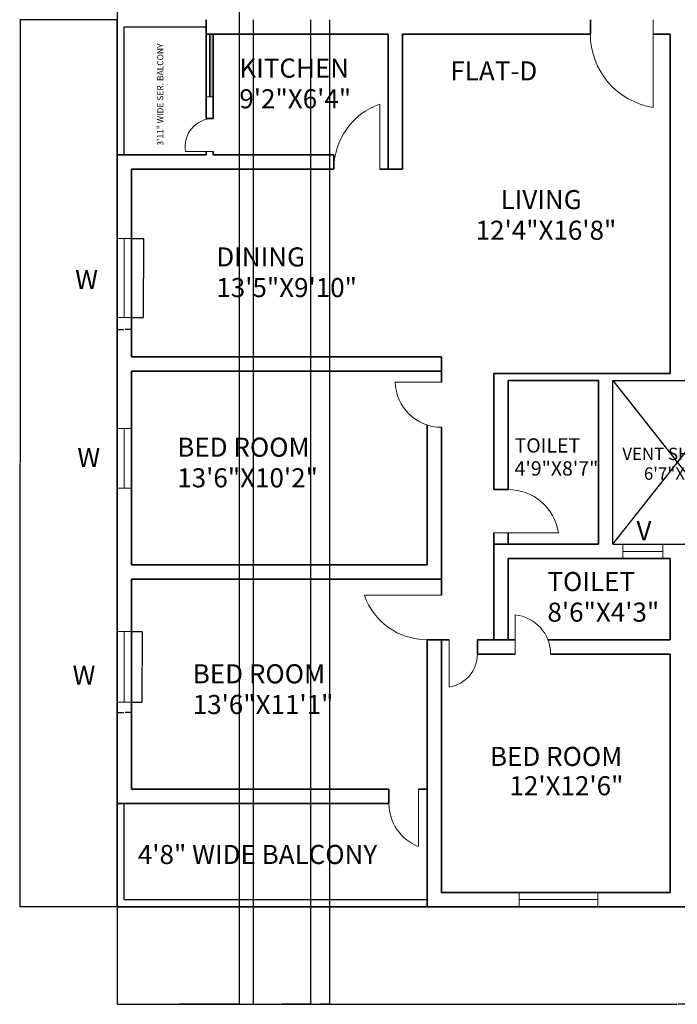
# Model space of a CAD drawing. Units: feet. Extents: x 5816 to 6644, y 25475 to 26788.
# Tile 1 of 23: x 5816 to 6230, y 25475 to 26094. Entities that reach past the tile are written whole.
import ezdxf

# ---------------------------------------------------------------- set-up
doc = ezdxf.new("R2010")
doc.units = ezdxf.units.FT
for name, color, linetype, lineweight in [('A-ANNO-DIMS', 2, 'Continuous', 13), ('A-ANNO-TEXT', 7, 'Continuous', 18), ('A-AREA-IDEN', 7, 'Continuous', 18), ('A-DOOR', 3, 'Continuous', 18), ('A-FLOR-RAIL', 8, 'Continuous', 25), ('A-FLOR-SHFT', 8, 'Continuous', 25), ('A-GLAZ', 4, 'Continuous', 18), ('A-WALL', 7, 'Continuous', 35)]:
    doc.layers.add(name, color=color, linetype=linetype, lineweight=lineweight)
doc.styles.get("Standard").update_dxf_attribs({"font": 'arial.ttf'})
doc.dimstyles.get("Standard").update_dxf_attribs({"dimtxt": 0.18, "dimasz": 0.18, "dimexe": 0.18, "dimexo": 0.0625, "dimgap": 0.09, "dimtad": 0, "dimtih": 1, "dimtoh": 1, "dimdec": 4, "dimzin": 0, "dimdsep": 46, "dimtxsty": 'Standard', "dimcen": 0.09, "dimadec": 0, "dimazin": 0, "dimtfac": 1, "dimtdec": 4, "dimtofl": 0, "dimtmove": 0, "dimatfit": 3, "dimfxl": 1, "dimtolj": 1, "dimtzin": 0, "dimarcsym": 0})

# ---------------------------------------------------------------- blocks, each defined once
blk = doc.blocks.new('DOOR-BALCONY')
blk.add_line((0, 36.11), (0, 0))
blk.add_arc((10.54, 9), 29.09, 111.24329, 180)
blk = doc.blocks.new('DOOR-BEDROOM-INNER')
blk.add_line((0, 29.82), (0, 0))
blk.add_arc((-3.45, 9), 21.11, 0, 80.59123)
blk = doc.blocks.new('DOOR-BEDROOM-BALCONY')
blk.add_line((-48.41, 0), (0, 0))
blk.add_arc((-9, -13.73), 41.74, 90, 160.78776)
blk = doc.blocks.new('DOOR-BEDROOM-SIDE')
blk.add_line((-28.98, 0), (0, 0))
blk.add_arc((0.03, -0.75), 29.02, 90, 178.52212)
blk = doc.blocks.new('DOOR-KITCHEN')
blk.add_line((0, -40.87), (0, 0))
blk.add_arc((14.45, 0), 43.35, 180, 250.52864)
blk = doc.blocks.new('DOOR-SERVICE-BALCONY')
blk.add_line((-17.56, 0), (0, 0))
blk.add_arc((0, -2.91), 17.8, 170.58679, 270)
blk = doc.blocks.new('DOOR-FLAT-ENTRY')
blk.add_line((0, 55.13), (0, 0))
blk.add_arc((7.05, 9.01), 46.66, 98.693, 180)
blk = doc.blocks.new('DOOR-BATH-ENSUITE')
blk.add_line((0, -24.59), (0, 0))
blk.add_arc((-2.33, 0.02), 24.72, 275.40734, 0)
blk = doc.blocks.new('DOOR-BATH-HALL')
blk.add_line((40.72, 0), (0, 0))
blk.add_arc((9, 4.86), 32.09, 270, 351.28818)
blk = doc.blocks.new('WIN-DINING')
for p, q in [((0, 0), (9, 0)), ((4.5, 0), (4.5, -49.84)), ((0, -49.84), (9, -49.84))]:
    blk.add_line(p, q)
blk = doc.blocks.new('WIN-BEDROOM-SIDE')
for p, q in [((0, 0), (9, 0)), ((4.5, 0), (4.5, -37.54)), ((0, -37.54), (9, -37.54))]:
    blk.add_line(p, q)
blk = doc.blocks.new('WIN-BEDROOM-BALCONY')
for p, q in [((0, 0), (9, 0)), ((4.5, 0), (4.5, -44.28)), ((0, -44.28), (9, -44.28))]:
    blk.add_line(p, q)
blk = doc.blocks.new('WIN-BEDROOM-INNER')
for p, q in [((49.5, 0), (49.5, -9)), ((0, 0), (0, -9)), ((0, -4.5), (49.5, -4.5))]:
    blk.add_line(p, q)
blk = doc.blocks.new('WIN-KITCHEN')
for p, q in [((0, 0), (4.5, 0)), ((2, 0), (2, -39.61)), ((3, 0), (3, -39.61))]:
    blk.add_line(p, q)
blk = doc.blocks.new('WIN-VENT-WIDE')
for p, q in [((0, 0), (0, -9)), ((0, -4.5), (25.2, -4.5)), ((25.2, 0), (25.2, -9))]:
    blk.add_line(p, q)
blk = doc.blocks.new('VENT-SHAFT')
for p, q in [((0, 0), (0, 103)), ((0, 103), (81, 103)), ((0, 103), (81, 0)), ((0, 0), (81, 103)), ((81, 103), (45, 103)), ((81, 0), (81, 103)), ((0, 0), (81, 0)), ((81, 0), (45, 0))]:
    blk.add_line(p, q)
blk = doc.blocks.new('RAIL-BALCONY-CORNER')
for p, q in [((0, 0), (0, -65)), ((0, 0), (195, 0)), ((4.5, -4.5), (4.5, -65)), ((4.5, -4.5), (195, -4.5))]:
    blk.add_line(p, q)
blk = doc.blocks.new('*D37')
at = {"layer": 'A-ANNO-DIMS', "color": 0, "lineweight": -2, "transparency": 16777216}
for p, q in [((5886.37, 25956.79), (5893.97, 25956.79)), ((5893.79, 25956.61), (5893.79, 25932.05)), ((5893.79, 25907.12), (5893.79, 25931.68)), ((5886.37, 25906.94), (5893.97, 25906.94))]:
    blk.add_line(p, q, dxfattribs=at)
at = {"layer": 'A-ANNO-DIMS', "color": 0, "transparency": 16777216}
for points in [[(5893.76, 25956.61), (5893.82, 25956.61), (5893.79, 25956.79)], [(5893.76, 25907.12), (5893.82, 25907.12), (5893.79, 25906.94)]]:
    blk.add_solid(points, dxfattribs=at)
at = {"layer": 'Defpoints', "color": 0, "transparency": 16777216}
for p in [(5886.31, 25956.79), (5886.31, 25906.94), (5893.79, 25906.94)]:
    blk.add_point(p, dxfattribs=at)
at = {"layer": 'A-ANNO-DIMS', "color": 0, "transparency": 16777216, "insert": (5893.79, 25931.86), "char_height": 0.18, "attachment_point": 5}
blk.add_mtext('\\A1;DINING WDW 50 TYP.', dxfattribs=at)
blk = doc.blocks.new('*D38')
at = {"layer": 'A-ANNO-DIMS', "color": 0, "lineweight": -2, "transparency": 16777216}
for p, q in [((5877.31, 25906.88), (5877.31, 25899.28)), ((5886.31, 25906.88), (5886.31, 25899.28)), ((5877.49, 25899.46), (5881.35, 25899.46)), ((5886.13, 25899.46), (5882.27, 25899.46))]:
    blk.add_line(p, q, dxfattribs=at)
at = {"layer": 'A-ANNO-DIMS', "color": 0, "transparency": 16777216}
for points in [[(5877.49, 25899.49), (5877.49, 25899.43), (5877.31, 25899.46)], [(5886.13, 25899.49), (5886.13, 25899.43), (5886.31, 25899.46)]]:
    blk.add_solid(points, dxfattribs=at)
at = {"layer": 'Defpoints', "color": 0, "transparency": 16777216}
for p in [(5877.31, 25906.94), (5886.31, 25906.94), (5877.31, 25899.46)]:
    blk.add_point(p, dxfattribs=at)
at = {"layer": 'A-ANNO-DIMS', "color": 0, "transparency": 16777216, "insert": (5881.81, 25899.46), "char_height": 0.18, "attachment_point": 5}
blk.add_mtext('\\A1;9 TYP.', dxfattribs=at)
blk = doc.blocks.new('*D41')
at = {"layer": 'A-ANNO-DIMS', "color": 0, "lineweight": -2, "transparency": 16777216}
for p, q in [((5886.37, 25709.41), (5893.13, 25709.41)), ((5892.95, 25709.23), (5892.95, 25687.45)), ((5892.95, 25665.31), (5892.95, 25687.09)), ((5886.37, 25665.13), (5893.13, 25665.13))]:
    blk.add_line(p, q, dxfattribs=at)
at = {"layer": 'A-ANNO-DIMS', "color": 0, "transparency": 16777216}
for points in [[(5892.92, 25709.23), (5892.98, 25709.23), (5892.95, 25709.41)], [(5892.92, 25665.31), (5892.98, 25665.31), (5892.95, 25665.13)]]:
    blk.add_solid(points, dxfattribs=at)
at = {"layer": 'Defpoints', "color": 0, "transparency": 16777216}
for p in [(5886.31, 25709.41), (5886.31, 25665.13), (5892.95, 25665.13)]:
    blk.add_point(p, dxfattribs=at)
at = {"layer": 'A-ANNO-DIMS', "color": 0, "transparency": 16777216, "insert": (5892.95, 25687.27), "char_height": 0.18, "attachment_point": 5}
blk.add_mtext('\\A1;BALCONY BR WDW 44 TYP.', dxfattribs=at)
blk = doc.blocks.new('*D42')
at = {"layer": 'A-ANNO-DIMS', "color": 0, "lineweight": -2, "transparency": 16777216}
for p, q in [((5877.31, 25665.07), (5877.31, 25658.31)), ((5886.31, 25665.07), (5886.31, 25658.31)), ((5877.49, 25658.49), (5881.35, 25658.49)), ((5886.13, 25658.49), (5882.27, 25658.49))]:
    blk.add_line(p, q, dxfattribs=at)
at = {"layer": 'A-ANNO-DIMS', "color": 0, "transparency": 16777216}
for points in [[(5877.49, 25658.52), (5877.49, 25658.46), (5877.31, 25658.49)], [(5886.13, 25658.52), (5886.13, 25658.46), (5886.31, 25658.49)]]:
    blk.add_solid(points, dxfattribs=at)
at = {"layer": 'Defpoints', "color": 0, "transparency": 16777216}
for p in [(5877.31, 25665.13), (5886.31, 25665.13), (5877.31, 25658.49)]:
    blk.add_point(p, dxfattribs=at)
at = {"layer": 'A-ANNO-DIMS', "color": 0, "transparency": 16777216, "insert": (5881.81, 25658.49), "char_height": 0.18, "attachment_point": 5}
blk.add_mtext('\\A1;9 TYP.', dxfattribs=at)
blk = doc.blocks.new('*D55')
at = {"layer": 'A-ANNO-DIMS', "color": 0, "lineweight": -2, "transparency": 16777216}
for p, q in [((5877.31, 25536.27), (5877.31, 25475.01)), ((6582.31, 25536.27), (6582.31, 25475.01)), ((5877.49, 25475.19), (6229.52, 25475.19)), ((6582.13, 25475.19), (6230.1, 25475.19))]:
    blk.add_line(p, q, dxfattribs=at)
at = {"layer": 'A-ANNO-DIMS', "color": 0, "transparency": 16777216}
for points in [[(5877.49, 25475.22), (5877.49, 25475.16), (5877.31, 25475.19)], [(6582.13, 25475.22), (6582.13, 25475.16), (6582.31, 25475.19)]]:
    blk.add_solid(points, dxfattribs=at)
at = {"layer": 'Defpoints', "color": 0, "transparency": 16777216}
for p in [(5877.31, 25536.34), (6582.31, 25536.34), (6582.31, 25475.19)]:
    blk.add_point(p, dxfattribs=at)
at = {"layer": 'A-ANNO-DIMS', "color": 0, "transparency": 16777216, "insert": (6229.81, 25475.19), "char_height": 0.18, "attachment_point": 5}
blk.add_mtext('\\A1;705', dxfattribs=at)
blk = doc.blocks.new('*D61')
at = {"layer": 'A-ANNO-DIMS', "color": 0, "lineweight": -2, "transparency": 16777216}
for p, q in [((5877.25, 26094.34), (5815.98, 26094.34)), ((5816.16, 26094.16), (5816.16, 25815.52)), ((5816.16, 25536.52), (5816.16, 25815.15)), ((5877.25, 25536.34), (5815.98, 25536.34))]:
    blk.add_line(p, q, dxfattribs=at)
at = {"layer": 'A-ANNO-DIMS', "color": 0, "transparency": 16777216}
for points in [[(5816.13, 26094.16), (5816.19, 26094.16), (5816.16, 26094.34)], [(5816.13, 25536.52), (5816.19, 25536.52), (5816.16, 25536.34)]]:
    blk.add_solid(points, dxfattribs=at)
at = {"layer": 'Defpoints', "color": 0, "transparency": 16777216}
for p in [(5816.16, 26094.34), (5877.31, 26094.34), (5877.31, 25536.34)]:
    blk.add_point(p, dxfattribs=at)
at = {"layer": 'A-ANNO-DIMS', "color": 0, "transparency": 16777216, "insert": (5816.16, 25815.34), "char_height": 0.18, "attachment_point": 5}
blk.add_mtext('\\A1;558', dxfattribs=at)
blk = doc.blocks.new('*D62')
at = {"layer": 'A-ANNO-DIMS', "color": 0, "lineweight": -2, "transparency": 16777216}
for p, q in [((5877.31, 26168.52), (5877.31, 25475.01)), ((5953.98, 26168.52), (5953.98, 25475.01)), ((5877.49, 25475.19), (5915.25, 25475.19)), ((5953.8, 25475.19), (5916.04, 25475.19))]:
    blk.add_line(p, q, dxfattribs=at)
at = {"layer": 'A-ANNO-DIMS', "color": 0, "transparency": 16777216}
for points in [[(5877.49, 25475.22), (5877.49, 25475.16), (5877.31, 25475.19)], [(5953.8, 25475.22), (5953.8, 25475.16), (5953.98, 25475.19)]]:
    blk.add_solid(points, dxfattribs=at)
at = {"layer": 'Defpoints', "color": 0, "transparency": 16777216}
for p in [(5877.31, 26168.58), (5953.98, 26168.58), (5953.98, 25475.19)]:
    blk.add_point(p, dxfattribs=at)
at = {"layer": 'A-ANNO-DIMS', "color": 0, "transparency": 16777216, "insert": (5915.64, 25475.19), "char_height": 0.18, "attachment_point": 5}
blk.add_mtext('\\A1;76.67', dxfattribs=at)
blk = doc.blocks.new('*D67')
at = {"layer": 'A-ANNO-DIMS', "color": 0, "lineweight": -2, "transparency": 16777216}
for p, q in [((5998.98, 26094.27), (5998.98, 25475.01)), ((6010.98, 26094.27), (6010.98, 25475.01)), ((5999.16, 25475.19), (6004.77, 25475.19)), ((6010.8, 25475.19), (6005.19, 25475.19))]:
    blk.add_line(p, q, dxfattribs=at)
at = {"layer": 'A-ANNO-DIMS', "color": 0, "transparency": 16777216}
for points in [[(5999.16, 25475.22), (5999.16, 25475.16), (5998.98, 25475.19)], [(6010.8, 25475.22), (6010.8, 25475.16), (6010.98, 25475.19)]]:
    blk.add_solid(points, dxfattribs=at)
at = {"layer": 'Defpoints', "color": 0, "transparency": 16777216}
for p in [(5998.98, 26094.34), (6010.98, 26094.34), (6010.98, 25475.19)]:
    blk.add_point(p, dxfattribs=at)
at = {"layer": 'A-ANNO-DIMS', "color": 0, "transparency": 16777216, "insert": (6004.98, 25475.19), "char_height": 0.18, "attachment_point": 5}
blk.add_mtext('\\A1;12', dxfattribs=at)
blk = doc.blocks.new('*D68')
at = {"layer": 'A-ANNO-DIMS', "color": 0, "lineweight": -2, "transparency": 16777216}
for p, q in [((5962.98, 26094.27), (5962.98, 25475.01)), ((5998.98, 26094.27), (5998.98, 25475.01)), ((5963.16, 25475.19), (5980.76, 25475.19)), ((5998.8, 25475.19), (5981.2, 25475.19))]:
    blk.add_line(p, q, dxfattribs=at)
at = {"layer": 'A-ANNO-DIMS', "color": 0, "transparency": 16777216}
for points in [[(5963.16, 25475.22), (5963.16, 25475.16), (5962.98, 25475.19)], [(5998.8, 25475.22), (5998.8, 25475.16), (5998.98, 25475.19)]]:
    blk.add_solid(points, dxfattribs=at)
at = {"layer": 'Defpoints', "color": 0, "transparency": 16777216}
for p in [(5962.98, 26094.34), (5998.98, 26094.34), (5998.98, 25475.19)]:
    blk.add_point(p, dxfattribs=at)
at = {"layer": 'A-ANNO-DIMS', "color": 0, "transparency": 16777216, "insert": (5980.98, 25475.19), "char_height": 0.18, "attachment_point": 5}
blk.add_mtext('\\A1;36', dxfattribs=at)

msp = doc.modelspace()

# ---------------------------------------------------------------- linework, layer by layer
at = {"layer": 'A-FLOR-RAIL'}
msp.add_lwpolyline([(5881.8119, 26009.3368), (5881.8119, 26089.8368), (5933.3119, 26089.8368)], dxfattribs=at)
at = {"layer": 'A-WALL'}
for p, q in [((5877.3119, 26000.3368), (5877.3119, 26094.3368)), ((5933.3119, 26032.2246), (5933.3119, 26094.3368)), ((6175.0829, 26085.3298), (6175.0829, 26094.3368)), ((5933.3119, 26085.3368), (6047.8119, 26085.3368)), ((5937.8119, 26032.2246), (5937.8119, 26085.3368)), ((6047.8119, 26085.3368), (6047.8119, 26000.3368)), ((6056.8119, 26085.3368), (6056.8119, 26009.3368)), ((6056.8119, 26085.3368), (6175.0829, 26085.3368)), ((6214.6905, 26085.3368), (6225.3119, 26085.3368)), ((6225.3119, 25871.8368), (6225.3119, 26085.3368)), ((5933.3119, 26032.2246), (5937.8119, 26032.2246)), ((5877.3119, 25610.3368), (5877.3119, 26009.3368)), ((5877.3119, 25751.3368), (5877.3119, 26009.3368)), ((5886.3119, 26009.3368), (5877.3119, 26009.3368)), ((5886.3119, 26009.3368), (5933.3119, 26009.3368)), ((5933.3119, 26009.3368), (5933.3119, 26011.5155)), ((5937.8119, 26009.3368), (5937.8119, 26011.5155)), ((5937.8119, 26009.3368), (6013.6326, 26009.3368)), ((6013.6326, 26000.3368), (6013.6326, 26009.3368)), ((6056.8119, 26009.3368), (6056.8119, 26000.3368)), ((5877.3119, 25882.3368), (5877.3119, 26000.3368)), ((5886.3119, 25882.3368), (5886.3119, 26000.3368)), ((5886.3119, 26000.3368), (6013.6326, 26000.3368)), ((6042.532, 26000.3368), (6056.8119, 26000.3368)), ((5886.3119, 25882.3368), (6081.3119, 25882.3368)), ((6081.3119, 25866.2444), (6081.3119, 25882.3368)), ((5886.3119, 25751.3368), (5886.3119, 25873.3368)), ((5886.3119, 25873.3368), (6081.3119, 25873.3368)), ((6114.3119, 25798.8236), (6114.3119, 25871.8368)), ((6123.3119, 25871.8368), (6114.3119, 25871.8368)), ((6123.3119, 25871.8368), (6225.3119, 25871.8368)), ((6123.3119, 25798.8236), (6123.3119, 25867.3368)), ((6123.3119, 25867.3368), (6180.3119, 25867.3368)), ((6180.3119, 25867.3368), (6180.3119, 25764.3368)), ((6072.3119, 25751.3368), (6072.3119, 25839.4181)), ((6081.3119, 25732.3387), (6081.3119, 25837.9771)), ((6123.3119, 25798.8236), (6114.3119, 25798.8236)), ((6114.3119, 25704.3368), (6114.3119, 25771.5927)), ((6123.3119, 25764.3368), (6123.3119, 25771.5927)), ((6114.3119, 25764.3368), (6180.3119, 25764.3368)), ((6123.3119, 25704.3368), (6123.3119, 25755.3368)), ((6123.3119, 25755.3368), (6225.3119, 25755.3368)), ((6225.3119, 25755.3368), (6225.3119, 25704.3368)), ((5886.3119, 25751.3368), (6072.3119, 25751.3368)), ((5886.3119, 25610.3368), (5886.3119, 25742.3368)), ((5886.3119, 25742.3368), (6081.3119, 25742.3368)), ((6081.3119, 25742.3368), (6081.3119, 25732.3387)), ((6086.3125, 25704.3368), (6072.3119, 25704.3368)), ((6072.3119, 25704.3368), (6072.3119, 25594.1569)), ((6081.3119, 25704.3368), (6081.3119, 25594.1569)), ((6127.6877, 25704.3368), (6103.9699, 25704.3368)), ((6103.9699, 25695.3368), (6103.9699, 25704.3368)), ((6127.6877, 25704.3368), (6123.3119, 25704.3368)), ((6225.3119, 25704.3368), (6148.3757, 25704.3368)), ((6225.3119, 25704.3368), (6148.3757, 25704.3368)), ((6127.6877, 25695.3368), (6103.9699, 25695.3368)), ((6225.3119, 25695.3368), (6150.0811, 25695.3368)), ((6225.3119, 25545.3368), (6225.3119, 25695.3368)), ((5877.3119, 25601.3368), (5877.3119, 25610.3368)), ((5886.3119, 25610.3368), (6048.3119, 25610.3368)), ((6048.3119, 25610.3368), (6048.3119, 25601.3368)), ((6066.8616, 25610.3368), (6072.3119, 25610.3368)), ((5877.3119, 25601.3368), (6048.3119, 25601.3368)), ((6072.3119, 25601.3368), (6072.3119, 25536.3368)), ((6081.3119, 25601.3368), (6081.3119, 25545.3368)), ((6081.3119, 25545.3368), (6225.3119, 25545.3368)), ((5877.3119, 25536.3368), (6279.7398, 25536.3368))]:
    msp.add_line(p, q, dxfattribs=at)

# ---------------------------------------------------------------- block references
at = {"layer": 'A-DOOR', "extrusion": (0, 0, -1), "zscale": -1, "rotation": 180}
for name, p in [('DOOR-FLAT-ENTRY', (-6214.6905, 26094.3368)), ('DOOR-KITCHEN', (-6042.532, 26000.3368)), ('DOOR-SERVICE-BALCONY', (-5937.8119, 26011.5155)), ('DOOR-BEDROOM-SIDE', (-6081.3119, 25866.2444)), ('DOOR-BATH-HALL', (-6114.3119, 25771.5927)), ('DOOR-BEDROOM-BALCONY', (-6081.3119, 25732.3387)), ('DOOR-BATH-ENSUITE', (-6127.6877, 25695.3368)), ('DOOR-BEDROOM-INNER', (-6086.3125, 25704.3368)), ('DOOR-BALCONY', (-6066.8616, 25610.3368))]:
    msp.add_blockref(name, p, dxfattribs=at)
at = {"layer": 'A-FLOR-RAIL', "extrusion": (0, 0, -1), "zscale": -1, "rotation": 180}
msp.add_blockref('RAIL-BALCONY-CORNER', (-5877.3119, 25536.3368), dxfattribs=at)
at = {"layer": 'A-FLOR-SHFT'}
msp.add_blockref('VENT-SHAFT', (6189.3119, 25764.3368), dxfattribs=at)
at = {"layer": 'A-GLAZ', "extrusion": (0, 0, -1), "zscale": -1, "rotation": 180}
msp.add_blockref('WIN-KITCHEN', (-5933.3119, 26045.731), dxfattribs=at)
at = {"layer": 'A-GLAZ', "rotation": 180}
for name, p in [('WIN-DINING', (5886.3119, 25906.9414)), ('WIN-VENT-WIDE', (6220.7941, 25755.3368)), ('WIN-BEDROOM-BALCONY', (5886.3119, 25665.1277)), ('WIN-BEDROOM-INNER', (6179.8839, 25536.3368))]:
    msp.add_blockref(name, p, dxfattribs=at)
at = {"layer": 'A-GLAZ'}
msp.add_blockref('WIN-BEDROOM-SIDE', (5877.3119, 25837.1796), dxfattribs=at)

# ---------------------------------------------------------------- texts
at = {"layer": 'A-ANNO-DIMS'}
for s, height, p in [('9\'2"X6\'4"', 12, (5954.1939, 26038.5936)), ('12\'4"X16\'8"', 12, (6102.9044, 25955.8889)), ('13\'5"X9\'10"', 12, (5939.6939, 25919.8346)), ('4\'9"X8\'7"', 8.98988, (6127.3994, 25807.605)), ('13\'6"X10\'2"', 12, (5915.1152, 25800.157)), ('6\'7"X8\'2"', 7.77416, (6208.7805, 25804.961)), ('8\'6"X4\'3"', 12, (6148.0836, 25715.6623)), ('13\'6"X11\'1"', 12, (5924.8804, 25657.6112)), ('12\'X12\'6"', 12, (6124.2051, 25606.4953))]:
    msp.add_text(s, height=height, dxfattribs=at).set_placement(p)
at = {"layer": 'A-ANNO-TEXT'}
for s, p in [('W', (5850.8604, 25924.9193)), ('W', (5852.2324, 25812.9842)), ('V', (6204.1133, 25766.9225)), ('W', (5849.2396, 25676.0869))]:
    msp.add_text(s, height=12, dxfattribs=at).set_placement(p)
at = {"layer": 'A-AREA-IDEN'}
msp.add_text('3\'11" WIDE SER. BALCONY', height=3.901456, rotation=90, dxfattribs=at).set_placement((5906.3672, 26015.0941))
for s, height, p in [('KITCHEN', 12, (5954.1939, 26057.8705)), ('FLAT-D', 12, (6087.0323, 26056.1209)), ('LIVING', 12, (6118.5941, 25975.1658)), ('DINING', 12, (5939.6939, 25939.1116)), ('BED ROOM', 12, (5915.1152, 25819.434)), ('TOILET', 8.98988, (6127.3994, 25822.0465)), ('VENT SHAFT', 7.77416, (6195.225, 25817.342)), ('TOILET', 12, (6148.0836, 25734.9392)), ('BED ROOM', 12, (5924.8804, 25676.8882)), ('BED ROOM', 12, (6111.9138, 25624.9252)), ('4\'8" WIDE BALCONY', 12, (5890.3368, 25563.2479))]:
    msp.add_text(s, height=height, dxfattribs=at).set_placement(p)

# ---------------------------------------------------------------- dimensions: what is measured, and where the dimension line sits
at = {"layer": 'A-ANNO-DIMS'}
for base, p1, p2, override, picture, middle in [((5953.9781, 25475.1868), (5877.3119, 26168.5846), (5953.9781, 26168.5846), {"dimdec": 2, "dimlfac": 1, "dimrnd": 0, "dimzin": 0, "dimdsep": 46, "dimlunit": 2}, '*D62', (5915.645, 25475.1868)), ((5998.9781, 25475.1868), (5962.9781, 26094.3368), (5998.9781, 26094.3368), {"dimdec": 0, "dimlfac": 1, "dimrnd": 0, "dimzin": 0, "dimdsep": 46, "dimlunit": 2}, '*D68', (5980.9781, 25475.1868)), ((6010.9781, 25475.1868), (5998.9781, 26094.3368), (6010.9781, 26094.3368), {"dimdec": 0, "dimlfac": 1, "dimrnd": 0, "dimzin": 0, "dimdsep": 46, "dimlunit": 2}, '*D67', (6004.9781, 25475.1868)), ((6582.3119, 25475.1868), (5877.3119, 25536.3368), (6582.3119, 25536.3368), {"dimdec": 0, "dimlfac": 1, "dimrnd": 0, "dimzin": 0, "dimdsep": 46, "dimlunit": 2}, '*D55', (6229.8119, 25475.1868))]:
    dim = msp.add_linear_dim(base=base, p1=p1, p2=p2, dimstyle='Standard', override=override, dxfattribs=at)
    dim.commit()
    dim.dimension.update_dxf_attribs({"geometry": picture, "text_midpoint": middle})
dim = msp.add_linear_dim(base=(5816.1619, 26094.3368), p1=(5877.3119, 25536.3368), p2=(5877.3119, 26094.3368), angle=90, dimstyle='Standard', override={"dimdec": 0, "dimlfac": 1, "dimrnd": 0, "dimzin": 0, "dimdsep": 46, "dimlunit": 2}, dxfattribs=at)
dim.commit()
dim.dimension.update_dxf_attribs({"geometry": '*D61', "text_midpoint": (5816.1619, 25815.3368)})
for base, p1, p2, angle, text, picture, middle in [((5893.7885, 25906.9414), (5886.3119, 25956.7857), (5886.3119, 25906.9414), 270, 'DINING WDW <> TYP.', '*D37', (5893.7885, 25931.8636)), ((5877.3119, 25899.4647), (5886.3119, 25906.9414), (5877.3119, 25906.9414), 180, '<> TYP.', '*D38', (5881.8119, 25899.4647)), ((5892.9542, 25665.1277), (5886.3119, 25709.4103), (5886.3119, 25665.1277), 270, 'BALCONY BR WDW <> TYP.', '*D41', (5892.9542, 25687.269)), ((5877.3119, 25658.4853), (5886.3119, 25665.1277), (5877.3119, 25665.1277), 180, '<> TYP.', '*D42', (5881.8119, 25658.4853))]:
    dim = msp.add_linear_dim(base=base, p1=p1, p2=p2, angle=angle, text=text, dimstyle='Standard', override={"dimdec": 0, "dimlfac": 1, "dimrnd": 0, "dimzin": 0, "dimdsep": 46, "dimlunit": 2}, dxfattribs=at)
    dim.commit()
    dim.dimension.update_dxf_attribs({"geometry": picture, "text_midpoint": middle})

doc.saveas('drawing.dxf')
